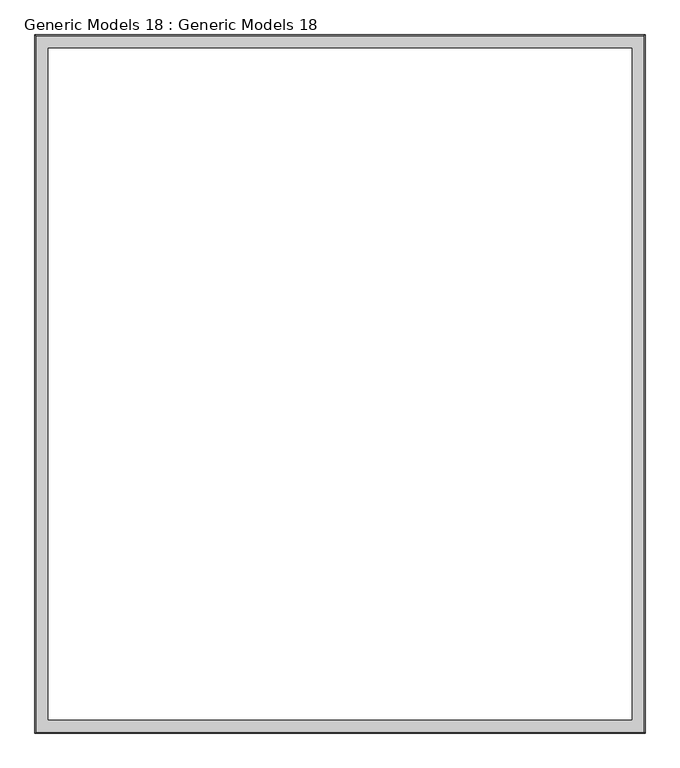
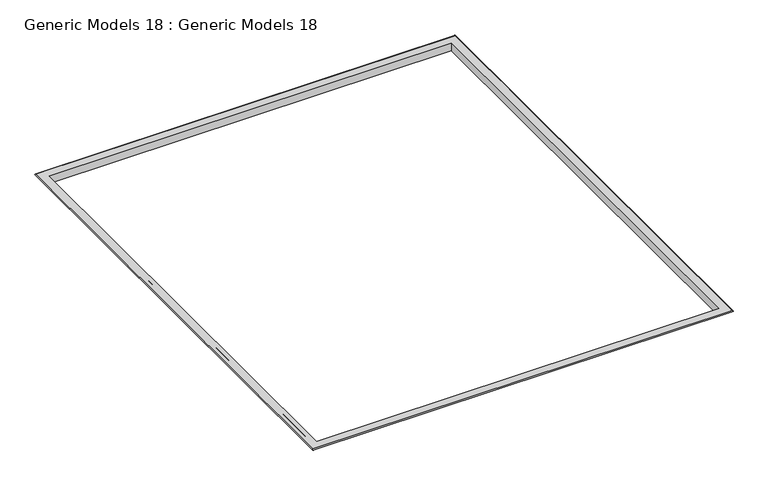
"""IFC4 building model written with IfcOpenShell, lengths in millimetres: proxy geometry, Generic Models 18 : Generic Models 18."""

from ifc_helpers import new_model, si_unit, frame, origin, place, context, project, spatial, polyline, ellipse_curve, source, transform, mapped, element, save
from ifc_brep_helpers import plane_surface, cylinder_surface, revolved_surface, advanced_brep


def generic_models_18_generic_models_18_23725794(model_context):
    return source(origin(), model_context, "Body", "AdvancedBrep", [
        advanced_brep(
        [(3818.6235854, -7475.3142532, 10668.0), (3818.6235854, -7475.3142532, 10972.8), (3818.6235854, 10386.9473869, 10972.8), (3818.6235854, 10386.9473869, 10668.0), (3996.4235854, -7653.1142532, 10820.4), (3996.4235854, 10564.7473869, 10820.4), (3996.4235854, -7653.1142532, 10871.2), (3996.4235854, 10564.7473869, 10871.2), (4072.6235854, -7729.3142532, 10922.0), (4072.6235854, -7729.3142532, 10871.2), (4072.6235854, 10640.9473869, 10871.2), (4072.6235854, 10640.9473869, 10922.0), (4148.8235854, -7805.5142532, 10972.8), (4148.8235854, -7805.5142532, 10922.0), (4148.8235854, 10717.1473869, 10922.0), (4148.8235854, 10717.1473869, 10972.8), (-11701.9275518, 10386.9473869, 10972.8), (-11701.9275518, 10386.9473869, 10668.0), (-11879.7275518, 10564.7473869, 10820.4), (-11879.7275518, 10564.7473869, 10871.2), (-11955.9275518, 10640.9473869, 10871.2), (-11955.9275518, 10640.9473869, 10922.0), (-12032.1275518, 10717.1473869, 10922.0), (-12032.1275518, 10717.1473869, 10972.8), (-11701.9275518, -7475.3142532, 10972.8), (-11701.9275518, -7475.3142532, 10668.0), (-11879.7275518, -7653.1142532, 10820.4), (-11879.7275518, -7653.1142532, 10871.2), (-11955.9275518, -7729.3142532, 10871.2), (-11955.9275518, -7729.3142532, 10922.0), (-12032.1275518, -7805.5142532, 10922.0), (-12032.1275518, -7805.5142532, 10972.8)],
        [
            (0, 1),
            (1, 2),
            (2, 3),
            (3, 0),
            (4, 0, ellipse_curve(frame((3991.9253088, -7648.6159766, 10645.7313227), z_axis=(-0.7071067811865475, -0.7071067811865475, 0.0), x_axis=(-0.7071067811865474, 0.7071067811865476, 0.0)), 247.1007135, 174.7265902)),
            (3, 5, ellipse_curve(frame((3991.9253088, 10560.2491103, 10645.7313227), z_axis=(-0.7071067811865475, 0.7071067811865475, 0.0), x_axis=(0.7071067811865474, 0.7071067811865476, 0.0)), 247.1007135, 174.7265902)),
            (5, 4),
            (6, 4),
            (5, 7),
            (7, 6),
            (8, 9),
            (9, 10),
            (10, 11),
            (11, 8),
            (12, 13, ellipse_curve(frame((4148.8235854, -7805.5142532, 10947.4), z_axis=(0.7071067811865475, 0.7071067811865475, 0.0), x_axis=(0.7071067811865474, -0.7071067811865476, 0.0)), 35.9210245, 25.4)),
            (13, 14),
            (14, 15, ellipse_curve(frame((4148.8235854, 10717.1473869, 10947.4), z_axis=(0.7071067811865475, -0.7071067811865475, 0.0), x_axis=(-0.7071067811865474, -0.7071067811865476, 0.0)), 35.9210245, 25.4)),
            (15, 12),
            (2, 16),
            (16, 17),
            (17, 3),
            (17, 18, ellipse_curve(frame((-11875.2292752, 10560.2491103, 10645.7313227), z_axis=(-0.7071067811865475, -0.7071067811865475, 0.0), x_axis=(-0.7071067811865476, 0.7071067811865474, 0.0)), 247.1007135, 174.7265902)),
            (18, 5),
            (18, 19),
            (19, 7),
            (10, 20),
            (20, 21),
            (21, 11),
            (14, 22),
            (22, 23, ellipse_curve(frame((-12032.1275518, 10717.1473869, 10947.4), z_axis=(0.7071067811865475, 0.7071067811865475, 0.0), x_axis=(0.7071067811865476, -0.7071067811865474, 0.0)), 35.9210245, 25.4)),
            (23, 15),
            (16, 24),
            (24, 25),
            (25, 17),
            (25, 26, ellipse_curve(frame((-11875.2292752, -7648.6159766, 10645.7313227), z_axis=(0.7071067811865475, -0.7071067811865475, 0.0), x_axis=(-0.7071067811865474, -0.7071067811865476, 0.0)), 247.1007135, 174.7265902)),
            (26, 18),
            (26, 27),
            (27, 19),
            (20, 28),
            (28, 29),
            (29, 21),
            (22, 30),
            (30, 31, ellipse_curve(frame((-12032.1275518, -7805.5142532, 10947.4), z_axis=(-0.7071067811865475, 0.7071067811865475, 0.0), x_axis=(0.7071067811865474, 0.7071067811865476, 0.0)), 35.9210245, 25.4)),
            (31, 23),
            (31, 12),
            (1, 24),
            (0, 25),
            (4, 26),
            (6, 27),
            (9, 28),
            (8, 29),
            (13, 30),
        ],
        [
            plane_surface(frame((3818.6235854, -7475.3142532, 10972.8), z_axis=(-1.0, 0.0, 0.0), x_axis=(0.0, 1.0, 0.0))),
            revolved_surface(polyline([(3817.1987186, 10734.975700451881, 10645.7313227), (3817.1987186, -7823.342566751884, 10645.7313227)]), (3991.9253088, -7475.3142532, 10645.7313227), (0.0, 1.0, 0.0)),
            plane_surface(frame((3996.4235854, -7653.1142532, 10820.4), z_axis=(1.0, 0.0, 0.0), x_axis=(0.0, 1.0, 0.0))),
            plane_surface(frame((4072.6235854, -7729.3142532, 10871.2), z_axis=(1.0, 0.0, 0.0), x_axis=(0.0, 1.0, 0.0))),
            cylinder_surface(frame((4148.8235854, -7475.3142532, 10947.4), z_axis=(0.0, -1.0, 0.0), x_axis=(-1.0, 0.0, 0.0)), 25.4),
            plane_surface(frame((3818.6235854, 10386.9473869, 10972.8), z_axis=(0.0, -1.0, 0.0), x_axis=(-1.0, 0.0, 0.0))),
            revolved_surface(polyline([(-12049.955865351883, 10385.5225201, 10645.7313227), (4166.6518989518845, 10385.5225201, 10645.7313227)]), (3818.6235854, 10560.2491103, 10645.7313227), (-1.0, 0.0, 0.0)),
            plane_surface(frame((3996.4235854, 10564.7473869, 10820.4), z_axis=(0.0, 1.0, 0.0), x_axis=(-1.0, 0.0, 0.0))),
            plane_surface(frame((4072.6235854, 10640.9473869, 10871.2), z_axis=(0.0, 1.0, 0.0), x_axis=(-1.0, 0.0, 0.0))),
            cylinder_surface(frame((3818.6235854, 10717.1473869, 10947.4), z_axis=(1.0, 0.0, 0.0), x_axis=(0.0, -1.0, 0.0)), 25.4),
            plane_surface(frame((-11701.9275518, 10386.9473869, 10972.8), z_axis=(1.0, 0.0, 0.0), x_axis=(0.0, -1.0, 0.0))),
            revolved_surface(polyline([(-11700.502685, -7823.342566751882, 10645.7313227), (-11700.502685, 10734.975700451883, 10645.7313227)]), (-11875.2292752, 10386.9473869, 10645.7313227), (0.0, -1.0, 0.0)),
            plane_surface(frame((-11879.7275518, 10564.7473869, 10820.4), z_axis=(-1.0, 0.0, 0.0), x_axis=(0.0, -1.0, 0.0))),
            plane_surface(frame((-11955.9275518, 10640.9473869, 10871.2), z_axis=(-1.0, 0.0, 0.0), x_axis=(0.0, -1.0, 0.0))),
            cylinder_surface(frame((-12032.1275518, 10386.9473869, 10947.4), z_axis=(0.0, 1.0, 0.0), x_axis=(1.0, 0.0, 0.0)), 25.4),
            plane_surface(frame((-12032.1275518, -7805.5142532, 10972.8), z_axis=(0.0, 0.0, 1.0), x_axis=(1.0, 0.0, 0.0))),
            plane_surface(frame((-11701.9275518, -7475.3142532, 10972.8), z_axis=(0.0, 1.0, 0.0), x_axis=(1.0, 0.0, 0.0))),
            revolved_surface(polyline([(4166.6518989518845, -7473.8893864, 10645.7313227), (-12049.955865351883, -7473.8893864, 10645.7313227)]), (-11701.9275518, -7648.6159766, 10645.7313227), (1.0, 0.0, 0.0)),
            plane_surface(frame((-11879.7275518, -7653.1142532, 10820.4), z_axis=(0.0, -1.0, 0.0), x_axis=(1.0, 0.0, 0.0))),
            plane_surface(frame((-11879.7275518, -7653.1142532, 10871.2), z_axis=(0.0, 0.0, -1.0), x_axis=(1.0, 0.0, 0.0))),
            plane_surface(frame((-11955.9275518, -7729.3142532, 10871.2), z_axis=(0.0, -1.0, 0.0), x_axis=(1.0, 0.0, 0.0))),
            plane_surface(frame((-11955.9275518, -7729.3142532, 10922.0), z_axis=(0.0, 0.0, -1.0), x_axis=(1.0, 0.0, 0.0))),
            cylinder_surface(frame((-11701.9275518, -7805.5142532, 10947.4), z_axis=(-1.0, 0.0, 0.0), x_axis=(0.0, 1.0, 0.0)), 25.4),
        ],
        [
            (0, [[1, 2, 3, 4]]),
            (1, [[5, -4, 6, 7]]),
            (2, [[8, -7, 9, 10]]),
            (3, [[11, 12, 13, 14]]),
            (4, [[15, 16, 17, 18]]),
            (5, [[-3, 19, 20, 21]]),
            (6, [[-6, -21, 22, 23]]),
            (7, [[-9, -23, 24, 25]]),
            (8, [[-13, 26, 27, 28]]),
            (9, [[-17, 29, 30, 31]]),
            (10, [[-20, 32, 33, 34]]),
            (11, [[-22, -34, 35, 36]]),
            (12, [[-24, -36, 37, 38]]),
            (13, [[-27, 39, 40, 41]]),
            (14, [[-30, 42, 43, 44]]),
            (15, [[-31, -44, 45, -18], [46, -32, -19, -2]]),
            (16, [[-33, -46, -1, 47]]),
            (17, [[-35, -47, -5, 48]]),
            (18, [[-37, -48, -8, 49]]),
            (19, [[50, -39, -26, -12], [-25, -38, -49, -10]]),
            (20, [[-40, -50, -11, 51]]),
            (21, [[52, -42, -29, -16], [-28, -41, -51, -14]]),
            (22, [[-43, -52, -15, -45]]),
        ],
    ),
    ])


if __name__ == "__main__":
    model = new_model("IFC4")
    model_context = context("Model", 3, world=origin())
    ifc_project = project(units=[si_unit("LENGTHUNIT", "METRE", prefix="MILLI")], contexts=[model_context])
    site = spatial("IfcSite", under=ifc_project)
    building = spatial("IfcBuilding", under=site)
    placement = place(None, origin())
    generic_models_18_generic_models_18_shape = generic_models_18_generic_models_18_23725794(model_context)
    element("IfcBuildingElementProxy", 1, Name="Generic Models 18 : Generic Models 18", ObjectType="Generic Models 18 : Generic Models 18", at=placement, inside=building, context=model_context, shape_type="MappedRepresentation", body=[
        mapped(generic_models_18_generic_models_18_shape, transform((0.0, 0.0, 0.0), x_axis=(1.0, 0.0, 0.0), y_axis=(0.0, 1.0, 0.0), z_axis=(0.0, 0.0, 1.0))),
    ])
    save(model, "model.ifc")
